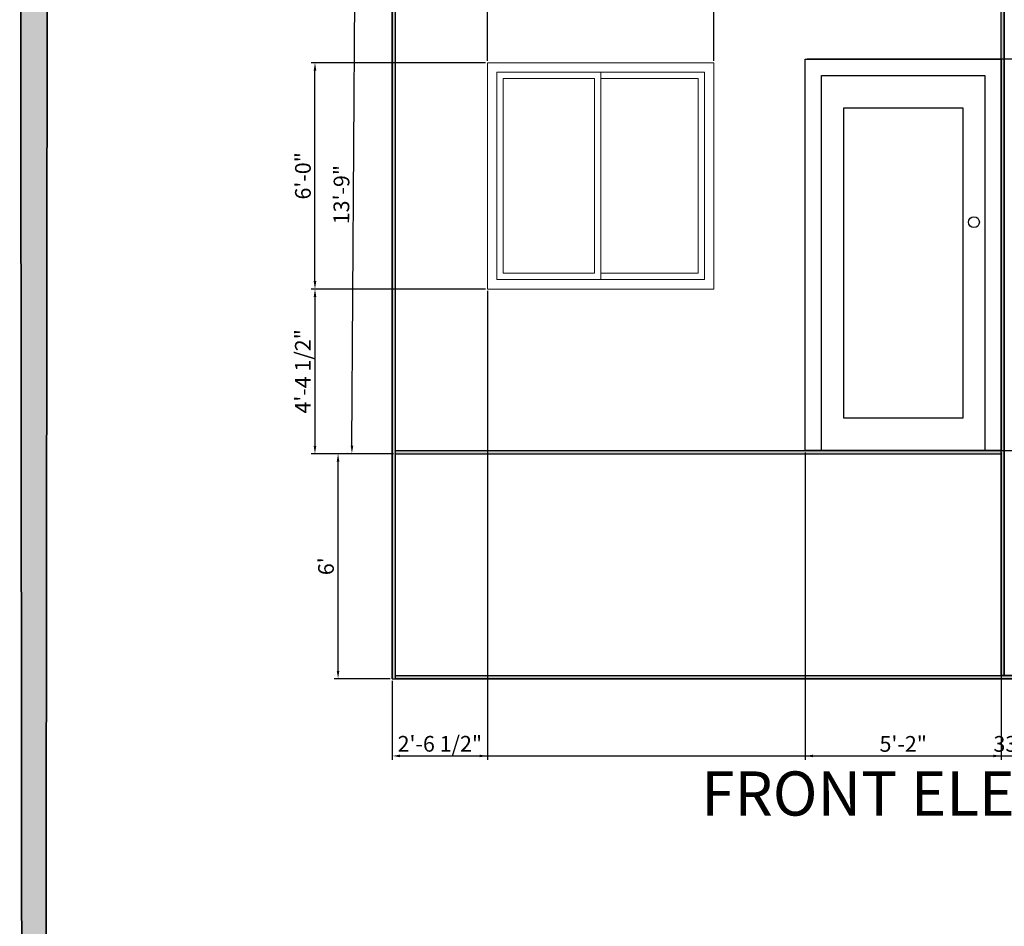
# Model space of a CAD drawing. Units: inches. Extents: x 1804 to 3296, y 909 to 2477.
# Tile 26 of 31: x 1804 to 2117, y 1900 to 2188. Entities that reach past the tile are written whole.
import ezdxf

# ---------------------------------------------------------------- set-up
doc = ezdxf.new("R2010")
doc.units = ezdxf.units.IN
for name, color, linetype, lineweight in [('A-ANNO-DIMS', 2, 'Continuous', 18), ('A-ANNO-TTLB', 156, 'Continuous', 35), ('A-ELEV-PATT', 85, 'Continuous', 13), ('A-WALL-PATT', 10, 'Continuous', 13), ('DOOR', 30, 'Continuous', 25), ('ELE', 210, 'Continuous', 30), ('TEXT', 190, 'Continuous', 18), ('WIND', 130, 'Continuous', 18)]:
    doc.layers.add(name, color=color, linetype=linetype, lineweight=lineweight)
doc.styles.get("Standard").update_dxf_attribs({"font": 'arial.ttf'})
doc.dimstyles.new('ISO-25', dxfattribs={"dimtxt": 5, "dimasz": 2.5, "dimexe": 1.25, "dimexo": 0.625, "dimtad": 1, "dimdec": 0, "dimlunit": 4, "dimtxsty": 'Standard', "dimcen": 2.5, "dimadec": 0, "dimazin": 0, "dimtfac": 1, "dimtdec": 0, "dimtmove": 0, "dimatfit": 3, "dimfxl": 1, "dimarcsym": 0})

# ---------------------------------------------------------------- blocks, each defined once
blk = doc.blocks.new('*U27')
blk.add_lwpolyline([(3.12, 0.01), (0.12, 0.01), (0.12, 72.01), (36.12, 72.01), (36.12, 0.01), (33.12, 0.01)])
for points in [[(33.12, 68.99), (33.12, 0.01), (3.12, 0.01), (3.12, 68.99)], [(29.12, 6.01), (29.12, 62.99), (7.12, 62.99), (7.12, 6.01)]]:
    blk.add_lwpolyline(points, close=True)
blk.add_circle((31.12, 42.01), 1)
blk = doc.blocks.new('*U24')
for p, q in [((1.5, 1.5), (1.5, 34.5)), ((1.5, 34.5), (18, 34.5)), ((18, 1.5), (18, 34.5)), ((18, 34.5), (34.5, 34.5)), ((34.5, 34.5), (34.5, 1.5)), ((18, 1.5), (1.5, 1.5)), ((34.5, 1.5), (18, 1.5))]:
    blk.add_line(p, q)
blk.add_lwpolyline([(0, 0), (0, 36), (36, 36), (36, 0)], close=True)
for points in [[(17, 33.5), (17, 2.5), (2.5, 2.5), (2.5, 33.5), (17, 33.5)], [(18, 33.5), (33.5, 33.5), (33.5, 2.5), (18, 2.5)]]:
    blk.add_lwpolyline(points)
blk = doc.blocks.new('*D28')
at = {"layer": 'A-ANNO-DIMS', "color": 0, "lineweight": -2, "transparency": 16777216}
for p, q in [((1921.54, 2050.31), (1903.7, 2050.31)), ((1904.95, 1981.29), (1904.95, 2047.81)), ((1921.54, 1978.79), (1903.7, 1978.79))]:
    blk.add_line(p, q, dxfattribs=at)
at = {"layer": 'A-ANNO-DIMS', "color": 0, "lineweight": 100, "transparency": 16777216}
for points in [[(1904.54, 2047.81), (1905.37, 2047.81), (1904.95, 2050.31)], [(1904.54, 1981.29), (1905.37, 1981.29), (1904.95, 1978.79)]]:
    blk.add_solid(points, dxfattribs=at)
at = {"layer": 'Defpoints', "color": 0, "lineweight": 100, "transparency": 16777216}
for p in [(1904.95, 2050.31), (1922.17, 2050.31), (1922.17, 1978.79)]:
    blk.add_point(p, dxfattribs=at)
at = {"layer": 'A-ANNO-DIMS', "color": 0, "transparency": 16777216, "insert": (1901.77, 2014.55), "char_height": 5, "attachment_point": 5, "rotation": 90}
blk.add_mtext("6'", dxfattribs=at)
blk = doc.blocks.new('*D29')
at = {"layer": 'A-ANNO-DIMS', "color": 0, "lineweight": -2, "transparency": 16777216}
for p, q in [((1922.54, 2214.87), (1909.11, 2214.95)), ((1909.37, 2052.89), (1910.34, 2212.44)), ((1921.54, 2050.32), (1908.11, 2050.4))]:
    blk.add_line(p, q, dxfattribs=at)
at = {"layer": 'A-ANNO-DIMS', "color": 0, "lineweight": 100, "transparency": 16777216}
for points in [[(1909.93, 2212.44), (1910.76, 2212.44), (1910.36, 2214.94)], [(1908.96, 2052.89), (1909.79, 2052.89), (1909.36, 2050.39)]]:
    blk.add_solid(points, dxfattribs=at)
at = {"layer": 'Defpoints', "color": 0, "lineweight": 100, "transparency": 16777216}
for p in [(1910.36, 2214.94), (1923.17, 2214.86), (1922.17, 2050.31)]:
    blk.add_point(p, dxfattribs=at)
at = {"layer": 'A-ANNO-DIMS', "color": 0, "transparency": 16777216, "insert": (1906.68, 2132.68), "char_height": 5, "attachment_point": 5, "rotation": 89.6518}
blk.add_mtext('13\'-9"', dxfattribs=at)
blk = doc.blocks.new('*D75')
at = {"layer": 'A-ANNO-DIMS', "color": 0, "lineweight": -2, "transparency": 16777216}
for p, q in [((1922.17, 1978.16), (1922.17, 1952.99)), ((2323.12, 1978.16), (2323.12, 1952.99)), ((1924.67, 1954.24), (2320.62, 1954.24))]:
    blk.add_line(p, q, dxfattribs=at)
at = {"layer": 'A-ANNO-DIMS', "color": 0, "lineweight": 100, "transparency": 16777216}
for points in [[(1924.67, 1954.65), (1924.67, 1953.82), (1922.17, 1954.24)], [(2320.62, 1954.65), (2320.62, 1953.82), (2323.12, 1954.24)]]:
    blk.add_solid(points, dxfattribs=at)
at = {"layer": 'Defpoints', "color": 0, "lineweight": 100, "transparency": 16777216}
for p in [(1922.17, 1978.79), (2323.12, 1978.79), (2323.12, 1954.24)]:
    blk.add_point(p, dxfattribs=at)
at = {"layer": 'A-ANNO-DIMS', "color": 0, "transparency": 16777216, "insert": (2122.65, 1957.42), "char_height": 5, "attachment_point": 5}
blk.add_mtext('33\'-5"', dxfattribs=at)
blk = doc.blocks.new('*D78')
at = {"layer": 'A-ANNO-DIMS', "color": 0, "lineweight": -2, "transparency": 16777216}
for p, q in [((1952.44, 2175.25), (1952.44, 2411.11)), ((1954.94, 2409.86), (2021.88, 2409.86)), ((2024.38, 2175.25), (2024.38, 2411.11))]:
    blk.add_line(p, q, dxfattribs=at)
at = {"layer": 'A-ANNO-DIMS', "color": 0, "lineweight": 100, "transparency": 16777216}
for points in [[(1954.94, 2410.28), (1954.94, 2409.44), (1952.44, 2409.86)], [(2021.88, 2410.28), (2021.88, 2409.44), (2024.38, 2409.86)]]:
    blk.add_solid(points, dxfattribs=at)
at = {"layer": 'Defpoints', "color": 0, "lineweight": 100, "transparency": 16777216}
for p in [(2024.38, 2409.86), (1952.44, 2174.63), (2024.38, 2174.63)]:
    blk.add_point(p, dxfattribs=at)
at = {"layer": 'A-ANNO-DIMS', "color": 0, "transparency": 16777216, "insert": (1988.41, 2413.04), "char_height": 5, "attachment_point": 5}
blk.add_mtext('6\'-0"', dxfattribs=at)
blk = doc.blocks.new('*D79')
at = {"layer": 'A-ANNO-DIMS', "color": 0, "lineweight": -2, "transparency": 16777216}
for p, q in [((1951.81, 2174.63), (1896.37, 2174.63)), ((1897.62, 2105.18), (1897.62, 2172.13)), ((1951.81, 2102.68), (1896.37, 2102.68))]:
    blk.add_line(p, q, dxfattribs=at)
at = {"layer": 'A-ANNO-DIMS', "color": 0, "lineweight": 100, "transparency": 16777216}
for points in [[(1897.2, 2172.13), (1898.04, 2172.13), (1897.62, 2174.63)], [(1897.2, 2105.18), (1898.04, 2105.18), (1897.62, 2102.68)]]:
    blk.add_solid(points, dxfattribs=at)
at = {"layer": 'Defpoints', "color": 0, "lineweight": 100, "transparency": 16777216}
for p in [(1897.62, 2174.63), (1952.44, 2174.63), (1952.44, 2102.68)]:
    blk.add_point(p, dxfattribs=at)
at = {"layer": 'A-ANNO-DIMS', "color": 0, "transparency": 16777216, "insert": (1894.44, 2138.66), "char_height": 5, "attachment_point": 5, "rotation": 90}
blk.add_mtext('6\'-0"', dxfattribs=at)
blk = doc.blocks.new('*D80')
at = {"layer": 'A-ANNO-DIMS', "color": 0, "lineweight": -2, "transparency": 16777216}
for p, q in [((1951.81, 2102.68), (1896.37, 2102.68)), ((1897.62, 2100.18), (1897.62, 2052.81)), ((1922.54, 2050.31), (1896.37, 2050.31))]:
    blk.add_line(p, q, dxfattribs=at)
at = {"layer": 'A-ANNO-DIMS', "color": 0, "lineweight": 100, "transparency": 16777216}
for points in [[(1897.2, 2100.18), (1898.04, 2100.18), (1897.62, 2102.68)], [(1897.2, 2052.81), (1898.04, 2052.81), (1897.62, 2050.31)]]:
    blk.add_solid(points, dxfattribs=at)
at = {"layer": 'Defpoints', "color": 0, "lineweight": 100, "transparency": 16777216}
for p in [(1952.44, 2102.68), (1897.62, 2050.31), (1923.17, 2050.31)]:
    blk.add_point(p, dxfattribs=at)
at = {"layer": 'A-ANNO-DIMS', "color": 0, "transparency": 16777216, "insert": (1894.41, 2076.5), "char_height": 5, "attachment_point": 5, "rotation": 90}
blk.add_mtext('4\'-4 1/2"', dxfattribs=at)
blk = doc.blocks.new('*D81')
at = {"layer": 'A-ANNO-DIMS', "color": 0, "lineweight": -2, "transparency": 16777216}
for p, q in [((1952.44, 2102.06), (1952.44, 1952.99)), ((1922.17, 1978.16), (1922.17, 1952.99)), ((1924.67, 1954.24), (1949.94, 1954.24))]:
    blk.add_line(p, q, dxfattribs=at)
at = {"layer": 'A-ANNO-DIMS', "color": 0, "lineweight": 100, "transparency": 16777216}
for points in [[(1924.67, 1954.65), (1924.67, 1953.82), (1922.17, 1954.24)], [(1949.94, 1954.65), (1949.94, 1953.82), (1952.44, 1954.24)]]:
    blk.add_solid(points, dxfattribs=at)
at = {"layer": 'Defpoints', "color": 0, "lineweight": 100, "transparency": 16777216}
for p in [(1952.44, 2102.68), (1922.17, 1978.79), (1952.44, 1954.24)]:
    blk.add_point(p, dxfattribs=at)
at = {"layer": 'A-ANNO-DIMS', "color": 0, "transparency": 16777216, "insert": (1937.3, 1957.45), "char_height": 5, "attachment_point": 5}
blk.add_mtext('2\'-6 1/2"', dxfattribs=at)
blk = doc.blocks.new('*D82')
at = {"layer": 'A-ANNO-DIMS', "color": 0, "lineweight": -2, "transparency": 16777216}
for p, q in [((2053.42, 2050.69), (2053.42, 1952.99)), ((2115.67, 2050.69), (2115.67, 1952.99)), ((2055.92, 1954.24), (2113.17, 1954.24))]:
    blk.add_line(p, q, dxfattribs=at)
at = {"layer": 'A-ANNO-DIMS', "color": 0, "lineweight": 100, "transparency": 16777216}
for points in [[(2055.92, 1954.65), (2055.92, 1953.82), (2053.42, 1954.24)], [(2113.17, 1954.65), (2113.17, 1953.82), (2115.67, 1954.24)]]:
    blk.add_solid(points, dxfattribs=at)
at = {"layer": 'Defpoints', "color": 0, "lineweight": 100, "transparency": 16777216}
for p in [(2053.42, 2051.31), (2115.67, 2051.31), (2115.67, 1954.24)]:
    blk.add_point(p, dxfattribs=at)
at = {"layer": 'A-ANNO-DIMS', "color": 0, "transparency": 16777216, "insert": (2084.55, 1957.42), "char_height": 5, "attachment_point": 5}
blk.add_mtext('5\'-2"', dxfattribs=at)
blk = doc.blocks.new('*D83')
at = {"layer": 'A-ANNO-DIMS', "color": 0, "lineweight": -2, "transparency": 16777216}
for p, q in [((2054.05, 2175.81), (2348.92, 2175.81)), ((2347.67, 2053.81), (2347.67, 2173.31)), ((2054.05, 2051.31), (2348.92, 2051.31))]:
    blk.add_line(p, q, dxfattribs=at)
at = {"layer": 'A-ANNO-DIMS', "color": 0, "lineweight": 100, "transparency": 16777216}
for points in [[(2347.26, 2173.31), (2348.09, 2173.31), (2347.67, 2175.81)], [(2347.26, 2053.81), (2348.09, 2053.81), (2347.67, 2051.31)]]:
    blk.add_solid(points, dxfattribs=at)
at = {"layer": 'Defpoints', "color": 0, "lineweight": 100, "transparency": 16777216}
for p in [(2053.42, 2175.81), (2347.67, 2175.81), (2053.42, 2051.31)]:
    blk.add_point(p, dxfattribs=at)
at = {"layer": 'A-ANNO-DIMS', "color": 0, "transparency": 16777216, "insert": (2344.46, 2113.56), "char_height": 5, "attachment_point": 5, "rotation": 90}
blk.add_mtext('10\'-4 1/2"', dxfattribs=at)

msp = doc.modelspace()

# ---------------------------------------------------------------- hatches: boundary and pattern name
at = {"layer": 'A-ANNO-TTLB'}
h = msp.add_hatch(color=256, dxfattribs=at)
h.dxf.hatch_style = 1
h.paths.add_polyline_path([(3294.53, 2476.54), (1803.79, 2476.54), (1805.43, 909.47), (3296.17, 909.47)])
h.paths.add_polyline_path([(1811, 914.33), (1812.79, 2467.54), (3285.53, 2467.54), (3283.74, 914.33)], flags=16)
h.paths.add_polyline_path([(1925.58, 1062.77), (1925.58, 1138.07), (1925.58, 1539.88), (1925.58, 1793.38), (1925.58, 1830.04), (2325.54, 1830.04), (2325.54, 1793.38), (2325.54, 1586.42), (2325.54, 1138.07), (2325.54, 1062.77)], flags=0)
h.paths.add_polyline_path([(1997.22, 1029.4), (2008.85, 1037.96), (2008.85, 1020.84)], flags=0)
h.paths.add_polyline_path([(1934.58, 1138.07), (1934.58, 1147.07), (2078.77, 1147.07), (2078.77, 1138.07), (2060.94, 1138.07)], flags=0)
h.paths.add_polyline_path([(1944.35, 1138.07), (1944.35, 1147.07), (2056.05, 1147.07), (2056.05, 1138.07)], flags=0)
h.paths.add_polyline_path([(2222.24, 1037.96), (2233.87, 1029.4), (2222.24, 1020.84)], flags=0)
h.paths.add_polyline_path([(2061.94, 1139.07), (2061.94, 1146.07), (2077.77, 1146.07), (2077.77, 1139.07)], flags=0)
h.paths.add_polyline_path([(2149.58, 1138.07), (2149.58, 1269.44), (2158.58, 1269.44), (2158.58, 1326.69), (2149.58, 1326.69), (2149.58, 1340.94), (2139.6, 1340.94), (2139.6, 1434.25), (2149.58, 1434.25), (2149.58, 1447.36), (2158.58, 1447.36), (2158.58, 1423.87), (2158.58, 1408.06), (2198.46, 1408.06), (2198.46, 1412.56), (2282.65, 1412.56), (2282.65, 1465.94), (2316.54, 1465.94), (2316.54, 1590.92), (2192.86, 1590.92), (2192.86, 1595.3), (2291.17, 1595.3), (2291.17, 1590.92), (2316.54, 1590.92), (2316.54, 1784.38), (2300.24, 1784.38), (2300.24, 1757.47), (2268, 1757.47), (2268, 1681.04), (2180.87, 1681.04), (2180.87, 1757.47), (2148.63, 1757.47), (2148.63, 1784.38), (2119.08, 1784.38), (2119.08, 1585.58), (2114.58, 1585.58), (2114.58, 1784.38), (2064.11, 1784.38), (2046.28, 1784.38), (2046.28, 1760.38), (1958.58, 1760.38), (1958.58, 1664.38), (1934.58, 1664.38), (1934.58, 1784.38), (1934.58, 1793.38), (2046.28, 1793.38), (2064.11, 1793.38), (2119.08, 1793.38), (2230.78, 1793.38), (2230.78, 1784.38), (2268, 1784.38), (2300.24, 1784.38), (2316.54, 1784.38), (2316.54, 1590.92), (2316.54, 1373.73), (2316.54, 1138.07)], flags=0)
h.paths.add_polyline_path([(2209.19, 1166.63), (2209.19, 1175.63), (2158.58, 1175.63), (2209.19, 1223.63), (2209.19, 1231.63), (2183.88, 1231.63), (2183.88, 1301.66), (2242.59, 1301.66), (2242.59, 1326.69), (2316.54, 1326.69), (2272.59, 1271.63), (2272.59, 1223.63), (2316.54, 1175.63), (2272.59, 1175.63), (2272.59, 1166.63)], flags=0)
h.paths.add_polyline_path([(1947.77, 1345.22), (1947.77, 1457.48), (1991.2, 1457.48), (1991.2, 1451.7), (1991.2, 1352.18), (1991.2, 1345.22)], flags=0)
h.paths.add_polyline_path([(2209.19, 1271.63), (2262.59, 1271.63), (2262.59, 1311.85), (2272.59, 1301.66), (2272.59, 1271.63), (2269.92, 1269.63), (2270.59, 1269.63), (2270.59, 1225.63), (2211.19, 1225.63), (2211.19, 1269.63), (2211.86, 1269.63)], flags=0)
h.paths.add_polyline_path([(2000.34, 1378.21), (2000.34, 1429.71), (2025.22, 1429.71), (2025.22, 1378.21)], flags=0)
h.paths.add_polyline_path([(2001.34, 1379.21), (2001.34, 1428.71), (2024.22, 1428.71), (2024.22, 1379.21)], flags=0)
h.paths.add_polyline_path([(2012.34, 1390.21), (2012.34, 1417.71), (2013.22, 1417.71), (2013.22, 1390.21)], flags=0)
h.paths.add_polyline_path([(2237.56, 1331.19), (2237.56, 1340.18), (2238.62, 1340.18), (2238.62, 1386.84), (2241.04, 1386.84), (2242.06, 1386.84), (2242.06, 1408.06), (2316.54, 1331.19)], flags=0)
h.paths.add_polyline_path([(1953.73, 1464.35), (1953.73, 1498.59), (1981.74, 1498.59), (1981.74, 1464.35)], flags=0)
h.paths.add_polyline_path([(1987.63, 1462.08), (1987.63, 1500.95), (2104.07, 1500.95), (2104.07, 1462.08), (2099.27, 1462.08), (1993.6, 1462.08)], flags=0)
h.paths.add_polyline_path([(1956.06, 1481.47, -1), (1979.41, 1481.47, -1)], flags=0)
edge = h.paths.add_edge_path(flags=0)
edge.add_ellipse((2299.53, 1438.37), major_axis=(0.31, 21.36), ratio=0.670333, start_angle=0, end_angle=360)
h.paths.add_polyline_path([(2297.39, 1438.37, -1), (2301.67, 1438.37, -1)], flags=0)
h.paths.add_polyline_path([(2591.54, 1163.23), (2591.54, 1179.38), (2591.54, 1379.68), (2591.54, 1395.84), (2734.5, 1395.84), (2734.5, 1379.68), (2734.5, 1179.38), (2734.5, 1163.23)], flags=0)
h.paths.add_polyline_path([(2592.54, 1164.23), (2592.54, 1166.23), (2733.5, 1166.23), (2733.5, 1164.23)], flags=0)
h.paths.add_polyline_path([(2592.54, 1180.38), (2592.54, 1378.68), (2733.5, 1378.68), (2733.5, 1180.38)], flags=0)
h.paths.add_polyline_path([(2593.54, 1181.38), (2593.54, 1377.68), (2732.5, 1377.68), (2732.5, 1181.38)], flags=0)
h.paths.add_polyline_path([(2594.54, 1182.38), (2594.54, 1376.68), (2731.5, 1376.68), (2731.5, 1182.38)], flags=0)
h.paths.add_polyline_path([(1936.95, 1697.46), (1936.95, 1736.46), (1955.41, 1736.46), (1955.41, 1697.46)], flags=0)
h.paths.add_polyline_path([(1938.48, 1718.36), (1938.48, 1734.92), (1953.65, 1734.92), (1953.65, 1718.36)], flags=0)
h.paths.add_polyline_path([(1944.75, 1726.64, -1), (1947.37, 1726.64, -1)], flags=0)
h.paths.add_polyline_path([(2592.54, 1394.84), (2733.5, 1394.84), (2733.5, 1392.84), (2592.54, 1392.84)], flags=0)
h.paths.add_polyline_path([(1976.61, 1762.5), (1976.61, 1781.44), (2012.79, 1781.44), (2012.79, 1762.5)], flags=0)
h.paths.add_polyline_path([(1979.57, 1771.97, -1), (1991.39, 1771.97, -1)], flags=0)
h.paths.add_polyline_path([(1995.36, 1771.97, -1), (2007.18, 1771.97, -1)], flags=0)
h.paths.add_polyline_path([(2251.51, 1744.53), (2268, 1730.05), (2251.51, 1730.05)], flags=0)
h.paths.add_polyline_path([(2047.28, 1785.38), (2047.28, 1792.38), (2063.11, 1792.38), (2063.11, 1785.38)], flags=0)
h.paths.add_polyline_path([(2155.08, 1770.92, -1), (2174.42, 1770.92, -1)], flags=0)
h.paths.add_polyline_path([(2188.59, 1758.27), (2188.59, 1772.81), (2222.3, 1772.81), (2222.3, 1758.27)], flags=0)
h.paths.add_polyline_path([(2223.97, 1758.27), (2223.97, 1772.81), (2257.68, 1772.81), (2257.68, 1758.27)], flags=0)
h.paths.add_polyline_path([(2274.45, 1770.92, -1), (2293.8, 1770.92, -1)], flags=0)
h.paths.add_polyline_path([(2591.54, 1582.09), (2591.54, 1782.39), (2734.5, 1782.39), (2734.5, 1582.09)], flags=0)
h.paths.add_polyline_path([(2592.54, 1583.09), (2592.54, 1781.39), (2733.5, 1781.39), (2733.5, 1583.09)], flags=0)
h.paths.add_polyline_path([(2593.54, 1584.09), (2593.54, 1780.39), (2732.5, 1780.39), (2732.5, 1584.09)], flags=0)
h.paths.add_polyline_path([(2594.54, 1585.09), (2594.54, 1779.39), (2731.5, 1779.39), (2731.5, 1585.09)], flags=0)
h.paths.add_polyline_path([(1922.17, 1978.79), (1922.17, 2295.08), (1922.17, 2296.08), (2115.67, 2296.08), (2115.67, 2384.31), (2115.67, 2385.31), (2322.12, 2385.31), (2323.12, 2385.31), (2323.12, 1979.79), (2323.12, 1978.79), (1923.17, 1978.79)], flags=0)
h.paths.add_polyline_path([(1922.17, 1978.79), (1922.17, 2051.31), (1922.17, 2214.86), (1922.17, 2296.08), (2115.67, 2296.08), (2115.67, 2385.31), (2323.12, 2385.31), (2323.12, 2280.42), (2323.12, 1978.79), (2115.67, 1978.79)], flags=0)
h.paths.add_polyline_path([(1923.17, 1979.79), (1923.17, 2050.31), (2115.67, 2050.31), (2115.67, 2051.31), (1923.17, 2051.31), (1923.17, 2213.86), (1923.17, 2214.86), (1923.17, 2295.08), (1990.02, 2295.08), (1990.02, 2214.86), (1991.02, 2214.86), (1991.02, 2295.08), (2115.67, 2295.08), (2115.67, 1979.79), (2116.67, 1979.79), (2116.67, 2304.18), (2116.67, 2384.31), (2322.12, 2384.31), (2322.12, 2280.42), (2322.12, 1979.79), (2115.67, 1979.79)], flags=0)
h.paths.add_polyline_path([(2972.46, 1192.5), (2972.46, 1196.92), (2995.47, 1196.92), (2995.47, 1255.47), (2995.09, 1255.47), (2987.42, 1249.39), (2980.08, 1255.47), (2978.05, 1255.47), (2978.05, 1257.24), (2995.47, 1257.24), (2995.47, 1261.58), (3015.37, 1261.58), (3015.37, 1333.28), (3015.37, 1414.4), (3032.82, 1414.4), (3032.82, 1333.28), (3032.82, 1261.58), (3052.66, 1261.58), (3052.66, 1255.47), (3079.86, 1255.47), (3078.72, 1254.57), (3081.47, 1252.29), (3078.56, 1249.99), (3075.81, 1252.26), (3072.57, 1249.69), (3070.36, 1251.52), (3067.67, 1249.39), (3060.34, 1255.47), (3052.66, 1255.47), (3052.66, 1196.92), (3054.58, 1196.92), (3074, 1196.92), (3074, 1192.5), (3052.66, 1192.5), (2995.47, 1192.5)], flags=0)
h.paths.add_polyline_path([(2490.75, 1979.27), (2490.75, 1980.27), (2596.87, 1980.27), (2596.87, 2051.8), (2596.87, 2052.8), (2596.87, 2216.35), (2596.87, 2297.57), (2717.32, 2297.57), (2710.57, 2305.62), (2724.07, 2305.62), (2717.32, 2297.57), (2782.37, 2297.57), (2782.37, 2395.8), (3006.82, 2395.8), (3006.82, 1981.27), (3093.73, 1981.27), (3093.73, 1980.27), (3047.51, 1980.27), (3046.37, 1979.37), (3049.11, 1977.1), (3046.2, 1974.79), (3043.46, 1977.07), (3040.21, 1974.49), (3038, 1976.32), (3035.32, 1974.2), (3027.98, 1980.27), (2871.83, 1980.27), (2871.83, 1981.27), (2791.37, 1981.27), (2791.37, 2050.8), (2597.87, 2050.8), (2597.87, 1980.27), (2597.87, 1979.27), (2546.27, 1979.27), (2545.12, 1978.37), (2547.87, 1976.1), (2544.96, 1973.79), (2542.22, 1976.07), (2538.97, 1973.49), (2536.76, 1975.32), (2534.07, 1973.2), (2526.74, 1979.27)], flags=0)
h.paths.add_polyline_path([(2597.87, 2051.8), (2606.87, 2051.8), (2606.87, 2258.39), (2597.87, 2258.39), (2597.87, 2296.57), (2606.87, 2296.57), (2606.87, 2262.39), (2782.37, 2262.39), (2782.37, 2296.57), (2790.37, 2296.57), (2790.37, 2262.39), (2791.37, 2262.39), (2791.37, 2305.67), (2791.37, 2385.8), (2996.82, 2385.8), (2996.82, 2339.85), (3006.82, 2339.85), (3006.82, 2250.12), (2997.82, 2250.12), (2997.82, 1981.27), (2996.82, 1981.27), (2872.83, 1981.27), (2872.83, 1991.8), (2871.83, 1991.8), (2871.83, 2050.8), (2790.37, 2050.8), (2597.87, 2050.8)], flags=0)
h.paths.add_polyline_path([(2179.93, 2153.92), (2179.93, 2353.97), (2259.98, 2353.97), (2259.98, 2153.92)], flags=0)
h.paths.add_polyline_path([(2180.93, 2154.92), (2180.93, 2352.97), (2258.98, 2352.97), (2258.98, 2154.92)], flags=0)
h.paths.add_polyline_path([(2960.87, 1608.49), (2960.87, 1753.62), (3070.9, 1753.62), (3070.9, 1608.49)], flags=0)
h.paths.add_polyline_path([(2961.87, 1609.49), (2961.87, 1752.62), (3069.9, 1752.62), (3069.9, 1609.49)], flags=0)
h.paths.add_polyline_path([(2962.87, 1610.49), (2962.87, 1751.62), (3068.9, 1751.62), (3068.9, 1610.49)], flags=0)
h.paths.add_polyline_path([(2963.87, 1611.49), (2963.87, 1750.62), (3067.9, 1750.62), (3067.9, 1611.49)], flags=0)
h.paths.add_polyline_path([(2782.37, 2051.8), (2782.37, 2216.32), (2791.37, 2216.32), (2791.37, 2051.8), (2872.83, 2051.8), (2872.83, 2068.56), (2884.67, 2068.56), (2884.67, 2085.33), (2896.51, 2085.33), (2896.51, 2102.09), (2908.36, 2102.09), (2908.36, 2118.85), (2920.2, 2118.85), (2920.2, 2135.62), (2932.05, 2135.62), (2932.05, 2145.3), (2925.08, 2145.3), (2925.08, 2203.2), (2996.82, 2203.2), (2996.82, 2145.3), (2953.82, 2145.3), (2872.83, 2051.8), (2790.37, 2051.8)], flags=0)
h.paths.add_polyline_path([(2717.32, 2238.65), (2710.57, 2246.7), (2724.07, 2246.7)], flags=0)
h.paths.add_polyline_path([(2003.09, 1122.79), (2017.16, 1122.79), (2017.16, 1138.74), (2003.09, 1138.74)], flags=8)
h.paths.add_polyline_path([(2174.76, 1792.72), (2188.83, 1792.72), (2188.83, 1808.66), (2174.76, 1808.66)], flags=8)
h.paths.add_polyline_path([(1987.95, 1792.51), (2002.02, 1792.51), (2002.02, 1808.45), (1987.95, 1808.45)], flags=8)
h.paths.add_polyline_path([(2148.79, 1289.26), (2160.46, 1289.26), (2160.46, 1305.2), (2148.79, 1305.2)], flags=8)
h.paths.add_polyline_path([(2115.36, 1133.57), (2127.04, 1133.57), (2127.04, 1149.51), (2115.36, 1149.51)], flags=8)
h.paths.add_polyline_path([(2237.58, 1421.48), (2249.25, 1421.48), (2249.25, 1437.43), (2237.58, 1437.43)], flags=8)
h.paths.add_polyline_path([(2134.99, 1584.32), (2146.66, 1584.32), (2146.66, 1600.26), (2134.99, 1600.26)], flags=8)
h.paths.add_polyline_path([(2101.95, 1557.31), (2113.62, 1557.31), (2113.62, 1573.25), (2101.95, 1573.25)], flags=8)
h.paths.add_polyline_path([(2937.85, 1156.77), (3120.41, 1156.77), (3120.41, 1185.72), (2937.85, 1185.72)], flags=8)
h.paths.add_polyline_path([(2980.71, 1786.71), (3050.06, 1786.71), (3050.06, 1802.66), (2980.71, 1802.66)], flags=8)
h.paths.add_polyline_path([(2869.28, 1661.96), (2938.62, 1661.96), (2938.62, 1690.8), (2869.28, 1690.8)], flags=8)
h.paths.add_polyline_path([(3092.27, 1674.86), (3161.62, 1674.86), (3161.62, 1690.8), (3092.27, 1690.8)], flags=8)
h.paths.add_polyline_path([(2980.71, 1674.86), (3050.06, 1674.86), (3050.06, 1690.8), (2980.71, 1690.8)], flags=8)
h.paths.add_polyline_path([(2649.07, 1678.23), (2674.53, 1678.23), (2674.53, 1714.76), (2649.07, 1714.76)], flags=8)
h.paths.add_polyline_path([(2530.84, 1981.63), (2549.13, 1981.63), (2549.13, 1997.57), (2530.84, 1997.57)], flags=8)
h.paths.add_polyline_path([(3031.29, 1981.77), (3049.58, 1981.77), (3049.58, 1997.71), (3031.29, 1997.71)], flags=8)
h.paths.add_polyline_path([(2715.38, 1911.9), (2851.54, 1911.9), (2851.54, 1940.85), (2715.38, 1940.85)], flags=8)
h.paths.add_polyline_path([(2015.23, 1927.36), (2205.42, 1927.36), (2205.42, 1956.3), (2015.23, 1956.3)], flags=8)
h.paths.add_polyline_path([(2671.84, 2057.84), (2702.75, 2057.84), (2702.75, 2073.79), (2671.84, 2073.79)], flags=8)
h.paths.add_polyline_path([(2678.5, 2316.52), (2765.26, 2316.52), (2765.26, 2332.46), (2678.5, 2332.46)], flags=8)
h.paths.add_polyline_path([(2678.48, 2271.96), (2736.41, 2271.96), (2736.41, 2287.9), (2678.48, 2287.9)], flags=8)
h.paths.add_polyline_path([(2019.2, 972.79), (2243.21, 972.79), (2243.21, 1001.74), (2019.2, 1001.74)], flags=8)
h.paths.add_polyline_path([(2097.06, 1021.56), (2132.16, 1021.56), (2132.16, 1037.51), (2097.06, 1037.51)], flags=8)
h.paths.add_polyline_path([(2182.47, 1360.48), (2207.35, 1360.48), (2207.35, 1376.42), (2182.47, 1376.42)], flags=8)
h.paths.add_polyline_path([(2261.12, 1361.77), (2295.01, 1361.77), (2295.01, 1377.71), (2261.12, 1377.71)], flags=8)
h.paths.add_polyline_path([(2245.75, 1511.51), (2278.44, 1511.51), (2278.44, 1527.46), (2245.75, 1527.46)], flags=8)
h.paths.add_polyline_path([(1991.16, 1296.29), (2060.51, 1296.29), (2060.51, 1312.23), (1991.16, 1312.23)], flags=8)
h.paths.add_polyline_path([(2187, 1651.35), (2246.71, 1651.35), (2246.71, 1667.29), (2187, 1667.29)], flags=8)
h.paths.add_polyline_path([(1976.49, 1684.81), (2068.63, 1684.81), (2068.63, 1700.76), (1976.49, 1700.76)], flags=8)
at = {"layer": 'A-ELEV-PATT'}
h = msp.add_hatch(color=256, dxfattribs=at)
h.dxf.hatch_style = 1
h.paths.add_polyline_path([(2116.67, 2384.31), (2115.67, 2384.31), (2115.67, 1979.79), (2116.67, 1979.79)])
h = msp.add_hatch(color=256, dxfattribs=at)
h.dxf.hatch_style = 1
h.paths.add_polyline_path([(1923.17, 2295.08), (1922.17, 2295.08), (1922.17, 1978.79), (1923.17, 1978.79)])
h = msp.add_hatch(color=256, dxfattribs=at)
h.dxf.hatch_style = 1
h.paths.add_polyline_path([(2115.67, 2051.31), (1923.17, 2051.31), (1923.17, 2050.31), (2115.67, 2050.31)])
h = msp.add_hatch(color=256, dxfattribs=at)
h.dxf.hatch_style = 1
h.paths.add_polyline_path([(2323.12, 1979.79), (1923.17, 1979.79), (1923.17, 1978.79), (2323.12, 1978.79)])
at = {"layer": 'A-WALL-PATT'}
h = msp.add_hatch(color=256, dxfattribs=at)
h.dxf.hatch_style = 1
h.paths.add_polyline_path([(2119.08, 1544.38), (1925.58, 1544.38), (1925.58, 1539.88), (2119.08, 1539.88)])
h.paths.add_polyline_path([(2119.08, 1545.58), (2114.58, 1545.58), (2114.58, 1544.38), (2119.08, 1544.38)])
h.paths.add_polyline_path([(1965.87, 1658.79), (1965.87, 1679.09), (1955.57, 1679.09), (1955.57, 1658.79)], flags=9)
h.paths.add_polyline_path([(2293.18, 1677.29), (2293.18, 1697.58), (2282.88, 1697.58), (2282.88, 1677.29)], flags=9)
h.paths.add_polyline_path([(2271.13, 1545.23), (2287.53, 1545.23), (2287.53, 1555.53), (2271.13, 1555.53)], flags=9)
h.paths.add_polyline_path([(2303.26, 1488.52), (2303.26, 1508.82), (2292.95, 1508.82), (2292.95, 1488.52)], flags=9)
h.paths.add_polyline_path([(2271.13, 1393.15), (2287.53, 1393.15), (2287.53, 1403.45), (2271.13, 1403.45)], flags=9)
h.paths.add_polyline_path([(2306.48, 1361.45), (2306.48, 1377.86), (2296.18, 1377.86), (2296.18, 1361.45)], flags=9)
h.paths.add_polyline_path([(2174.54, 1361.45), (2174.54, 1377.86), (2164.23, 1377.86), (2164.23, 1361.45)], flags=9)
h.paths.add_polyline_path([(1968.21, 1333.34), (1968.21, 1353.64), (1957.91, 1353.64), (1957.91, 1333.34)], flags=9)
h.paths.add_polyline_path([(2003.09, 1122.79), (2017.16, 1122.79), (2017.16, 1138.74), (2003.09, 1138.74)], flags=9)
h.paths.add_polyline_path([(2174.76, 1792.72), (2188.83, 1792.72), (2188.83, 1808.66), (2174.76, 1808.66)], flags=9)
h.paths.add_polyline_path([(1987.95, 1792.51), (2002.02, 1792.51), (2002.02, 1808.45), (1987.95, 1808.45)], flags=9)
h.paths.add_polyline_path([(2148.79, 1289.26), (2160.46, 1289.26), (2160.46, 1305.2), (2148.79, 1305.2)], flags=9)
h.paths.add_polyline_path([(2115.36, 1133.57), (2127.04, 1133.57), (2127.04, 1149.51), (2115.36, 1149.51)], flags=9)
h.paths.add_polyline_path([(2237.58, 1421.48), (2249.25, 1421.48), (2249.25, 1437.43), (2237.58, 1437.43)], flags=9)
h.paths.add_polyline_path([(2134.99, 1584.32), (2146.66, 1584.32), (2146.66, 1600.26), (2134.99, 1600.26)], flags=9)
h.paths.add_polyline_path([(2101.95, 1557.31), (2113.62, 1557.31), (2113.62, 1573.25), (2101.95, 1573.25)], flags=9)
h.paths.add_polyline_path([(2937.85, 1156.77), (3120.41, 1156.77), (3120.41, 1185.72), (2937.85, 1185.72)], flags=9)
h.paths.add_polyline_path([(2980.71, 1786.71), (3050.06, 1786.71), (3050.06, 1802.66), (2980.71, 1802.66)], flags=9)
h.paths.add_polyline_path([(2869.28, 1661.96), (2938.62, 1661.96), (2938.62, 1690.8), (2869.28, 1690.8)], flags=9)
h.paths.add_polyline_path([(3092.27, 1674.86), (3161.62, 1674.86), (3161.62, 1690.8), (3092.27, 1690.8)], flags=9)
h.paths.add_polyline_path([(2980.71, 1674.86), (3050.06, 1674.86), (3050.06, 1690.8), (2980.71, 1690.8)], flags=9)
h.paths.add_polyline_path([(2649.07, 1678.23), (2674.53, 1678.23), (2674.53, 1714.76), (2649.07, 1714.76)], flags=9)
h.paths.add_polyline_path([(2530.84, 1981.63), (2549.13, 1981.63), (2549.13, 1997.57), (2530.84, 1997.57)], flags=9)
h.paths.add_polyline_path([(3031.29, 1981.77), (3049.58, 1981.77), (3049.58, 1997.71), (3031.29, 1997.71)], flags=9)
h.paths.add_polyline_path([(2715.38, 1911.9), (2851.54, 1911.9), (2851.54, 1940.85), (2715.38, 1940.85)], flags=9)
h.paths.add_polyline_path([(2015.23, 1927.36), (2205.42, 1927.36), (2205.42, 1956.3), (2015.23, 1956.3)], flags=9)
h.paths.add_polyline_path([(2671.84, 2057.84), (2702.75, 2057.84), (2702.75, 2073.79), (2671.84, 2073.79)], flags=9)
h.paths.add_polyline_path([(2678.5, 2316.52), (2765.26, 2316.52), (2765.26, 2332.46), (2678.5, 2332.46)], flags=9)
h.paths.add_polyline_path([(2678.48, 2271.96), (2736.41, 2271.96), (2736.41, 2287.9), (2678.48, 2287.9)], flags=9)
h.paths.add_polyline_path([(2019.2, 972.79), (2243.21, 972.79), (2243.21, 1001.74), (2019.2, 1001.74)], flags=9)
h.paths.add_polyline_path([(2097.06, 1021.56), (2132.16, 1021.56), (2132.16, 1037.51), (2097.06, 1037.51)], flags=9)
h.paths.add_polyline_path([(2182.47, 1360.48), (2207.35, 1360.48), (2207.35, 1376.42), (2182.47, 1376.42)], flags=9)
h.paths.add_polyline_path([(2261.12, 1361.77), (2295.01, 1361.77), (2295.01, 1377.71), (2261.12, 1377.71)], flags=9)
h.paths.add_polyline_path([(2245.75, 1511.51), (2278.44, 1511.51), (2278.44, 1527.46), (2245.75, 1527.46)], flags=9)
h.paths.add_polyline_path([(1991.16, 1296.29), (2060.51, 1296.29), (2060.51, 1312.23), (1991.16, 1312.23)], flags=9)
h.paths.add_polyline_path([(2187, 1651.35), (2246.71, 1651.35), (2246.71, 1667.29), (2187, 1667.29)], flags=9)
h.paths.add_polyline_path([(1976.49, 1684.81), (2068.63, 1684.81), (2068.63, 1700.76), (1976.49, 1700.76)], flags=9)
h = msp.add_hatch(color=256, dxfattribs=at)
h.dxf.hatch_style = 1
h.paths.add_polyline_path([(2149.58, 1147.07), (2141.21, 1147.07), (2141.21, 1144.07), (2141.21, 1138.07), (2149.58, 1138.07)])
h.paths.add_polyline_path([(2101.21, 1144.07, -0.01877), (2101.32, 1147.07), (2078.77, 1147.07), (2078.77, 1138.07), (2101.21, 1138.07)])
h.paths.add_polyline_path([(2060.94, 1147.07), (2056.05, 1147.07), (2056.05, 1138.07), (2060.94, 1138.07)])
h.paths.add_polyline_path([(1944.35, 1147.07), (1934.58, 1147.07), (1934.58, 1138.07), (1944.35, 1138.07)])
h.paths.add_polyline_path([(2158.58, 1269.44), (2149.58, 1269.44), (2149.58, 1138.07), (2158.58, 1138.07)])
h.paths.add_polyline_path([(2003.09, 1122.79), (2017.16, 1122.79), (2017.16, 1138.74), (2003.09, 1138.74)], flags=9)
h.paths.add_polyline_path([(2174.76, 1792.72), (2188.83, 1792.72), (2188.83, 1808.66), (2174.76, 1808.66)], flags=9)
h.paths.add_polyline_path([(1987.95, 1792.51), (2002.02, 1792.51), (2002.02, 1808.45), (1987.95, 1808.45)], flags=9)
h.paths.add_polyline_path([(2148.79, 1289.26), (2160.46, 1289.26), (2160.46, 1305.2), (2148.79, 1305.2)], flags=9)
h.paths.add_polyline_path([(2115.36, 1133.57), (2127.04, 1133.57), (2127.04, 1149.51), (2115.36, 1149.51)], flags=9)
h.paths.add_polyline_path([(2237.58, 1421.48), (2249.25, 1421.48), (2249.25, 1437.43), (2237.58, 1437.43)], flags=9)
h.paths.add_polyline_path([(2134.99, 1584.32), (2146.66, 1584.32), (2146.66, 1600.26), (2134.99, 1600.26)], flags=9)
h.paths.add_polyline_path([(2101.95, 1557.31), (2113.62, 1557.31), (2113.62, 1573.25), (2101.95, 1573.25)], flags=9)
h.paths.add_polyline_path([(2937.85, 1156.77), (3120.41, 1156.77), (3120.41, 1185.72), (2937.85, 1185.72)], flags=9)
h.paths.add_polyline_path([(2980.71, 1786.71), (3050.06, 1786.71), (3050.06, 1802.66), (2980.71, 1802.66)], flags=9)
h.paths.add_polyline_path([(2869.28, 1661.96), (2938.62, 1661.96), (2938.62, 1690.8), (2869.28, 1690.8)], flags=9)
h.paths.add_polyline_path([(3092.27, 1674.86), (3161.62, 1674.86), (3161.62, 1690.8), (3092.27, 1690.8)], flags=9)
h.paths.add_polyline_path([(2980.71, 1674.86), (3050.06, 1674.86), (3050.06, 1690.8), (2980.71, 1690.8)], flags=9)
h.paths.add_polyline_path([(2649.07, 1678.23), (2674.53, 1678.23), (2674.53, 1714.76), (2649.07, 1714.76)], flags=9)
h.paths.add_polyline_path([(2530.84, 1981.63), (2549.13, 1981.63), (2549.13, 1997.57), (2530.84, 1997.57)], flags=9)
h.paths.add_polyline_path([(3031.29, 1981.77), (3049.58, 1981.77), (3049.58, 1997.71), (3031.29, 1997.71)], flags=9)
h.paths.add_polyline_path([(2715.38, 1911.9), (2851.54, 1911.9), (2851.54, 1940.85), (2715.38, 1940.85)], flags=9)
h.paths.add_polyline_path([(2015.23, 1927.36), (2205.42, 1927.36), (2205.42, 1956.3), (2015.23, 1956.3)], flags=9)
h.paths.add_polyline_path([(2671.84, 2057.84), (2702.75, 2057.84), (2702.75, 2073.79), (2671.84, 2073.79)], flags=9)
h.paths.add_polyline_path([(2678.5, 2316.52), (2765.26, 2316.52), (2765.26, 2332.46), (2678.5, 2332.46)], flags=9)
h.paths.add_polyline_path([(2678.48, 2271.96), (2736.41, 2271.96), (2736.41, 2287.9), (2678.48, 2287.9)], flags=9)
h.paths.add_polyline_path([(2019.2, 972.79), (2243.21, 972.79), (2243.21, 1001.74), (2019.2, 1001.74)], flags=9)
h.paths.add_polyline_path([(2097.06, 1021.56), (2132.16, 1021.56), (2132.16, 1037.51), (2097.06, 1037.51)], flags=9)
h.paths.add_polyline_path([(2182.47, 1360.48), (2207.35, 1360.48), (2207.35, 1376.42), (2182.47, 1376.42)], flags=9)
h.paths.add_polyline_path([(2261.12, 1361.77), (2295.01, 1361.77), (2295.01, 1377.71), (2261.12, 1377.71)], flags=9)
h.paths.add_polyline_path([(2245.75, 1511.51), (2278.44, 1511.51), (2278.44, 1527.46), (2245.75, 1527.46)], flags=9)
h.paths.add_polyline_path([(1991.16, 1296.29), (2060.51, 1296.29), (2060.51, 1312.23), (1991.16, 1312.23)], flags=9)
h.paths.add_polyline_path([(2187, 1651.35), (2246.71, 1651.35), (2246.71, 1667.29), (2187, 1667.29)], flags=9)
h.paths.add_polyline_path([(1976.49, 1684.81), (2068.63, 1684.81), (2068.63, 1700.76), (1976.49, 1700.76)], flags=9)
h = msp.add_hatch(color=256, dxfattribs=at)
h.dxf.hatch_style = 1
h.paths.add_polyline_path([(2158.58, 1275.49), (2155.29, 1275.49), (2149.58, 1275.49), (2149.58, 1269.44), (2158.58, 1269.44)])
h.paths.add_polyline_path([(2158.58, 1326.69), (2149.58, 1326.69), (2149.58, 1319.33), (2155.29, 1319.33), (2158.58, 1319.33)])
h.paths.add_polyline_path([(2158.58, 1402.2), (2158.58, 1423.87), (2158.58, 1447.36), (2149.58, 1447.36), (2149.58, 1423.87), (2149.58, 1340.94), (2149.58, 1326.69), (2158.58, 1326.69), (2158.58, 1354.23)])
h.paths.add_polyline_path([(1965.87, 1658.79), (1965.87, 1679.09), (1955.57, 1679.09), (1955.57, 1658.79)], flags=9)
h.paths.add_polyline_path([(2293.18, 1677.29), (2293.18, 1697.58), (2282.88, 1697.58), (2282.88, 1677.29)], flags=9)
h.paths.add_polyline_path([(2271.13, 1545.23), (2287.53, 1545.23), (2287.53, 1555.53), (2271.13, 1555.53)], flags=9)
h.paths.add_polyline_path([(2303.26, 1488.52), (2303.26, 1508.82), (2292.95, 1508.82), (2292.95, 1488.52)], flags=9)
h.paths.add_polyline_path([(2271.13, 1393.15), (2287.53, 1393.15), (2287.53, 1403.45), (2271.13, 1403.45)], flags=9)
h.paths.add_polyline_path([(2306.48, 1361.45), (2306.48, 1377.86), (2296.18, 1377.86), (2296.18, 1361.45)], flags=9)
h.paths.add_polyline_path([(2189.9, 1340.62), (2206.31, 1340.62), (2206.31, 1350.92), (2189.9, 1350.92)], flags=9)
h.paths.add_polyline_path([(2174.54, 1361.45), (2174.54, 1377.86), (2164.23, 1377.86), (2164.23, 1361.45)], flags=9)
h.paths.add_polyline_path([(2304.24, 1240.8), (2304.24, 1261.09), (2293.94, 1261.09), (2293.94, 1240.8)], flags=9)
h.paths.add_polyline_path([(2227.19, 1188.73), (2247.49, 1188.73), (2247.49, 1199.03), (2227.19, 1199.03)], flags=9)
h.paths.add_polyline_path([(2181.93, 1144.21), (2181.93, 1160.62), (2171.63, 1160.62), (2171.63, 1144.21)], flags=9)
h.paths.add_polyline_path([(1968.21, 1333.34), (1968.21, 1353.64), (1957.91, 1353.64), (1957.91, 1333.34)], flags=9)
h.paths.add_polyline_path([(2029.78, 1203.53), (2053.95, 1203.53), (2053.95, 1213.83), (2029.78, 1213.83)], flags=9)
h.paths.add_polyline_path([(2576.51, 1671.88), (2576.51, 1692.17), (2566.21, 1692.17), (2566.21, 1671.88)], flags=9)
h.paths.add_polyline_path([(2566.99, 1269.67), (2566.99, 1289.96), (2556.68, 1289.96), (2556.68, 1269.67)], flags=9)
h.paths.add_polyline_path([(2581.85, 1269.17), (2581.85, 1289.46), (2571.54, 1289.46), (2571.54, 1269.17)], flags=9)
h.paths.add_polyline_path([(2650.71, 1409.75), (2674.89, 1409.75), (2674.89, 1420.05), (2650.71, 1420.05)], flags=9)
h.paths.add_polyline_path([(2003.09, 1122.79), (2017.16, 1122.79), (2017.16, 1138.74), (2003.09, 1138.74)], flags=9)
h.paths.add_polyline_path([(2174.76, 1792.72), (2188.83, 1792.72), (2188.83, 1808.66), (2174.76, 1808.66)], flags=9)
h.paths.add_polyline_path([(1987.95, 1792.51), (2002.02, 1792.51), (2002.02, 1808.45), (1987.95, 1808.45)], flags=9)
h.paths.add_polyline_path([(2148.79, 1289.26), (2160.46, 1289.26), (2160.46, 1305.2), (2148.79, 1305.2)], flags=9)
h.paths.add_polyline_path([(2115.36, 1133.57), (2127.04, 1133.57), (2127.04, 1149.51), (2115.36, 1149.51)], flags=9)
h.paths.add_polyline_path([(2237.58, 1421.48), (2249.25, 1421.48), (2249.25, 1437.43), (2237.58, 1437.43)], flags=9)
h.paths.add_polyline_path([(2134.99, 1584.32), (2146.66, 1584.32), (2146.66, 1600.26), (2134.99, 1600.26)], flags=9)
h.paths.add_polyline_path([(2101.95, 1557.31), (2113.62, 1557.31), (2113.62, 1573.25), (2101.95, 1573.25)], flags=9)
h.paths.add_polyline_path([(2937.85, 1156.77), (3120.41, 1156.77), (3120.41, 1185.72), (2937.85, 1185.72)], flags=9)
h.paths.add_polyline_path([(2980.71, 1786.71), (3050.06, 1786.71), (3050.06, 1802.66), (2980.71, 1802.66)], flags=9)
h.paths.add_polyline_path([(2869.28, 1661.96), (2938.62, 1661.96), (2938.62, 1690.8), (2869.28, 1690.8)], flags=9)
h.paths.add_polyline_path([(3092.27, 1674.86), (3161.62, 1674.86), (3161.62, 1690.8), (3092.27, 1690.8)], flags=9)
h.paths.add_polyline_path([(2980.71, 1674.86), (3050.06, 1674.86), (3050.06, 1690.8), (2980.71, 1690.8)], flags=9)
h.paths.add_polyline_path([(2649.07, 1678.23), (2674.53, 1678.23), (2674.53, 1714.76), (2649.07, 1714.76)], flags=9)
h.paths.add_polyline_path([(2530.84, 1981.63), (2549.13, 1981.63), (2549.13, 1997.57), (2530.84, 1997.57)], flags=9)
h.paths.add_polyline_path([(3031.29, 1981.77), (3049.58, 1981.77), (3049.58, 1997.71), (3031.29, 1997.71)], flags=9)
h.paths.add_polyline_path([(2715.38, 1911.9), (2851.54, 1911.9), (2851.54, 1940.85), (2715.38, 1940.85)], flags=9)
h.paths.add_polyline_path([(2015.23, 1927.36), (2205.42, 1927.36), (2205.42, 1956.3), (2015.23, 1956.3)], flags=9)
h.paths.add_polyline_path([(2671.84, 2057.84), (2702.75, 2057.84), (2702.75, 2073.79), (2671.84, 2073.79)], flags=9)
h.paths.add_polyline_path([(2678.5, 2316.52), (2765.26, 2316.52), (2765.26, 2332.46), (2678.5, 2332.46)], flags=9)
h.paths.add_polyline_path([(2678.48, 2271.96), (2736.41, 2271.96), (2736.41, 2287.9), (2678.48, 2287.9)], flags=9)
h.paths.add_polyline_path([(2019.2, 972.79), (2243.21, 972.79), (2243.21, 1001.74), (2019.2, 1001.74)], flags=9)
h.paths.add_polyline_path([(2097.06, 1021.56), (2132.16, 1021.56), (2132.16, 1037.51), (2097.06, 1037.51)], flags=9)
h.paths.add_polyline_path([(2182.47, 1360.48), (2207.35, 1360.48), (2207.35, 1376.42), (2182.47, 1376.42)], flags=9)
h.paths.add_polyline_path([(2261.12, 1361.77), (2295.01, 1361.77), (2295.01, 1377.71), (2261.12, 1377.71)], flags=9)
h.paths.add_polyline_path([(2245.75, 1511.51), (2278.44, 1511.51), (2278.44, 1527.46), (2245.75, 1527.46)], flags=9)
h.paths.add_polyline_path([(1991.16, 1296.29), (2060.51, 1296.29), (2060.51, 1312.23), (1991.16, 1312.23)], flags=9)
h.paths.add_polyline_path([(2187, 1651.35), (2246.71, 1651.35), (2246.71, 1667.29), (2187, 1667.29)], flags=9)
h.paths.add_polyline_path([(1976.49, 1684.81), (2068.63, 1684.81), (2068.63, 1700.76), (1976.49, 1700.76)], flags=9)

# ---------------------------------------------------------------- linework, layer by layer
at = {"layer": 'A-ANNO-TTLB'}
for points in [[(1803.79, 2476.54), (3294.53, 2476.54), (3296.17, 909.47), (1805.43, 909.47)], [(1812.79, 2467.54), (3285.53, 2467.54), (3283.74, 914.33), (1811, 914.33)]]:
    msp.add_lwpolyline(points, close=True, dxfattribs=at)
at = {"layer": 'ELE'}
for p, q in [((2116.67, 1979.79), (2116.67, 2304.18)), ((2115.67, 1979.79), (2115.67, 2295.08)), ((1922.17, 2051.31), (1922.17, 2214.86)), ((1923.17, 2051.31), (1923.17, 2213.86)), ((1922.17, 1978.79), (1922.17, 2051.31)), ((1923.17, 2051.31), (2115.67, 2051.31)), ((1923.17, 1979.79), (1923.17, 2050.31)), ((1923.17, 2050.31), (2115.67, 2050.31)), ((1922.17, 1978.79), (2115.67, 1978.79)), ((1923.17, 1979.79), (2115.67, 1979.79)), ((2115.67, 1979.79), (2322.12, 1979.79)), ((2115.67, 1978.79), (2323.12, 1978.79))]:
    msp.add_line(p, q, dxfattribs=at)
for points in [[(2115.67, 2384.31), (2116.67, 2384.31), (2116.67, 1979.79), (2115.67, 1979.79)], [(1922.17, 1978.79), (1923.17, 1978.79), (1923.17, 2295.08), (1922.17, 2295.08)], [(2323.12, 1978.79), (1923.17, 1978.79), (1923.17, 1979.79), (2323.12, 1979.79)]]:
    msp.add_lwpolyline(points, close=True, dxfattribs=at)
for points in [[(2227.37, 1979.79), (2115.67, 1979.79)], [(2227.37, 1978.79), (2115.67, 1978.79)]]:
    msp.add_lwpolyline(points, dxfattribs=at)

# ---------------------------------------------------------------- block references
at = {"layer": 'DOOR', "xscale": 1.72916268390833, "yscale": 1.72916268390833, "zscale": 1.72916268390833}
msp.add_blockref('*U27', (2053.21, 2051.29), dxfattribs=at)
at = {"layer": 'WIND', "xscale": 1.99847867905339, "yscale": 1.99847867905339, "zscale": 1.99847867905339}
msp.add_blockref('*U24', (1952.44, 2102.68), dxfattribs=at)

# ---------------------------------------------------------------- texts
at = {"layer": 'TEXT', "insert": (2020.35, 1949.32), "char_height": 14.0468, "attachment_point": 1}
msp.add_mtext_dynamic_manual_height_columns('FRONT ELEVATION', width=296.512, gutter_width=70.23, heights=[0], dxfattribs=at)

# ---------------------------------------------------------------- dimensions: what is measured, and where the dimension line sits
at = {"layer": 'A-ANNO-DIMS'}
for base, p1, p2, picture, middle in [((2024.38, 2409.86), (1952.44, 2174.63), (2024.38, 2174.63), '*D78', (1988.41, 2413.04)), ((1952.44, 1954.24), (1922.17, 1978.79), (1952.44, 2102.68), '*D81', (1937.3, 1957.45)), ((2115.6699, 1954.2374), (2053.4201, 2051.3138), (2115.6699, 2051.3138), '*D82', (2084.545, 1957.4153)), ((2323.1246, 1954.2374), (1922.1699, 1978.7874), (2323.1246, 1978.7874), '*D75', (2122.6473, 1957.417))]:
    dim = msp.add_linear_dim(base=base, p1=p1, p2=p2, dimstyle='ISO-25', override={"dimdec": 1, "dimlfac": 1, "dimrnd": 0, "dimzin": 1, "dimdsep": 46, "dimlunit": 4, "dimfrac": 2}, dxfattribs=at)
    dim.commit()
    dim.dimension.update_dxf_attribs({"geometry": picture, "text_midpoint": middle})
dim = msp.add_aligned_dim(p1=(1922.17, 2050.31), p2=(1923.17, 2214.86), distance=12.81, dimstyle='ISO-25', override={"dimclrd": 0, "dimclre": 0, "dimclrt": 0}, dxfattribs=at)
dim.commit()
dim.dimension.update_dxf_attribs({"geometry": '*D29', "text_midpoint": (1906.68, 2132.68)})
for base, p1, p2, override, picture, middle in [((1897.6199, 2174.629), (1952.4367, 2102.6838), (1952.4367, 2174.629), {"dimdec": 1, "dimlfac": 1, "dimrnd": 0, "dimzin": 1, "dimdsep": 46, "dimlunit": 4, "dimfrac": 2}, '*D79', (1894.4421, 2138.6564)), ((2347.67, 2175.81), (2053.42, 2051.31), (2053.42, 2175.81), {"dimdec": 1, "dimlfac": 1, "dimrnd": 0, "dimzin": 1, "dimdsep": 46, "dimlunit": 4, "dimfrac": 2}, '*D83', (2344.46, 2113.56)), ((1897.62, 2050.31), (1952.44, 2102.68), (1923.17, 2050.31), {"dimdec": 1, "dimlfac": 1, "dimrnd": 0, "dimzin": 1, "dimdsep": 46, "dimlunit": 4, "dimfrac": 2}, '*D80', (1894.41, 2076.5)), ((1904.95, 2050.31), (1922.17, 1978.79), (1922.17, 2050.31), {"dimclrd": 0, "dimclre": 0, "dimclrt": 0}, '*D28', (1901.77, 2014.55))]:
    dim = msp.add_linear_dim(base=base, p1=p1, p2=p2, angle=90, dimstyle='ISO-25', override=override, dxfattribs=at)
    dim.commit()
    dim.dimension.update_dxf_attribs({"geometry": picture, "text_midpoint": middle})

doc.saveas('drawing.dxf')
